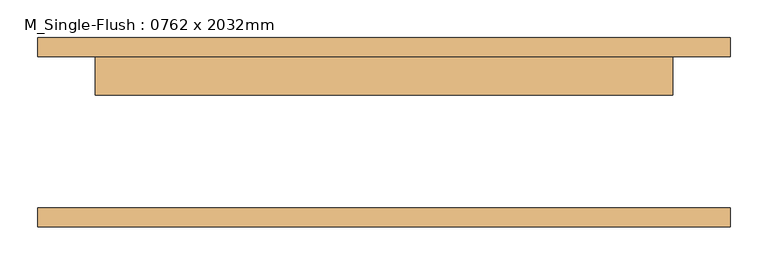
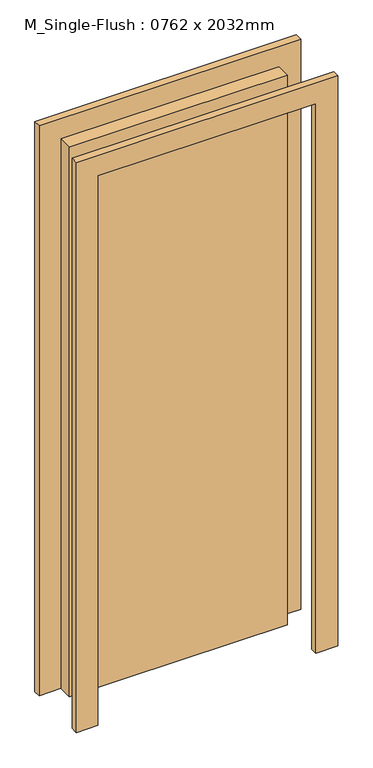
"""IFC4 building model written with IfcOpenShell, lengths in millimetres: door geometry, M_Single-Flush : 0762 x 2032mm."""

from ifc_helpers import new_model, si_unit, frame, origin, origin_with_axes, place, context, project, spatial, polyline, outline, extrude, source, transform, mapped, element, save


def m_single_flush_0762_x_2032mm_0c256fab(model_context):
    return source(origin(), model_context, "Body", "SweptSolid", [
        extrude(outline(polyline([(2108.0, -457.0), (0.0, -457.0), (0.0, -381.0), (2032.0, -381.0), (2032.0, 381.0), (0.0, 381.0), (0.0, 457.0), (2108.0, 457.0), (2108.0, -457.0)])), frame((0.0, 100.0, 0.0), z_axis=(0.0, 1.0, 0.0), x_axis=(0.0, 0.0, 1.0)), (0.0, 0.0, 1.0), 25.0),
        extrude(outline(polyline([(2108.0, 457.0), (2108.0, -457.0), (0.0, -457.0), (0.0, -381.0), (2032.0, -381.0), (2032.0, 381.0), (0.0, 381.0), (0.0, 457.0), (2108.0, 457.0)])), frame((0.0, -125.0, 0.0), z_axis=(0.0, 1.0, 0.0), x_axis=(0.0, 0.0, 1.0)), (0.0, 0.0, 1.0), 25.0),
        extrude(outline(polyline([(381.0, 49.0), (-381.0, 49.0), (-381.0, 100.0), (381.0, 100.0), (381.0, 49.0)])), origin_with_axes(), (0.0, 0.0, 1.0), 2032.0),
    ])


if __name__ == "__main__":
    model = new_model("IFC4")
    model_context = context("Model", 3, world=origin())
    ifc_project = project(units=[si_unit("LENGTHUNIT", "METRE", prefix="MILLI")], contexts=[model_context])
    site = spatial("IfcSite", under=ifc_project)
    building = spatial("IfcBuilding", under=site)
    placement = place(None, origin())
    m_single_flush_0762_x_2032mm_shape = m_single_flush_0762_x_2032mm_0c256fab(model_context)
    element("IfcDoor", 1, ObjectType="M_Single-Flush : 0762 x 2032mm", at=placement, inside=building, context=model_context, shape_type="MappedRepresentation", body=[
        mapped(m_single_flush_0762_x_2032mm_shape, transform((0.0, 0.0, 0.0), x_axis=(1.0, 0.0, 0.0), y_axis=(0.0, 1.0, 0.0), z_axis=(0.0, 0.0, 1.0))),
    ])
    save(model, "model.ifc")

# Revit data of these elements
# Type "M_Single-Flush : 0762 x 2032mm"
#   Type Mark = "19"
#   Thickness = 51 mm
#   Height = 2032 mm
#   Trim Projection Ext = 25 mm
#   Trim Projection Int = 25 mm
#   Trim Width = 76 mm
#   Width = 762 mm
#   Door Material = Door - Panel
#   Frame Material = Door - Frame
#   Function = (empty or 0)
#   Wall Closure = (empty or 0)
# Element 1 (IfcDoor, "M_Single-Flush : 0762 x 2032mm")
#   Materials on its faces: "Door - Frame", "Door - Panel"
# Materials
#   "Door - Panel": class "Wood", colour RGB 114 82 51, transparency 0
#   "Door - Frame": colour RGB 153 76 43, transparency 0
